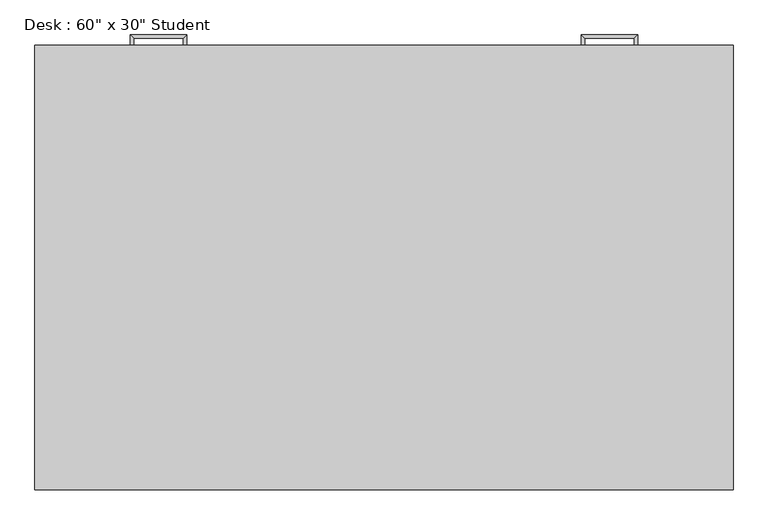
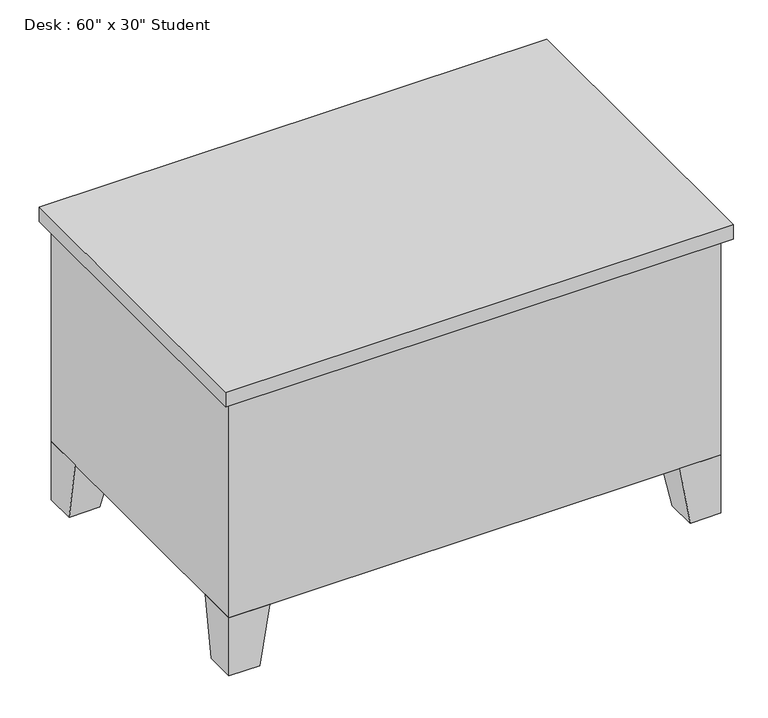
"""IFC4 building model written with IfcOpenShell, lengths in millimetres: furniture geometry."""

from ifc_helpers import new_model, si_unit, frame, origin, place, context, project, spatial, polyline, outline, extrude, faceted_brep, source, transform, mapped, element, save


def furniture_8768a1f0(model_context):
    return source(origin(), model_context, "Body", "SolidModel", [
        extrude(outline(polyline([(1200.15, 762.0), (831.85, 762.0), (831.85, 774.7), (1200.15, 774.7), (1200.15, 762.0)])), frame((0.0, 0.0, 603.25), z_axis=(0.0, 0.0, 1.0), x_axis=(1.0, 0.0, 0.0)), (0.0, 0.0, 1.0), 101.6),
        extrude(outline(polyline([(1200.15, 762.0), (831.85, 762.0), (831.85, 774.7), (1200.15, 774.7), (1200.15, 762.0)])), frame((0.0, 0.0, 171.45), z_axis=(0.0, 0.0, 1.0), x_axis=(1.0, 0.0, 0.0)), (0.0, 0.0, 1.0), 412.75),
        extrude(outline(polyline([(387.35, 762.0), (19.05, 762.0), (19.05, 774.7), (387.35, 774.7), (387.35, 762.0)])), frame((0.0, 0.0, 603.25), z_axis=(0.0, 0.0, 1.0), x_axis=(1.0, 0.0, 0.0)), (0.0, 0.0, 1.0), 101.6),
        extrude(outline(polyline([(387.35, 762.0), (19.05, 762.0), (19.05, 774.7), (387.35, 774.7), (387.35, 762.0)])), frame((0.0, 0.0, 171.45), z_axis=(0.0, 0.0, 1.0), x_axis=(1.0, 0.0, 0.0)), (0.0, 0.0, 1.0), 171.45),
        extrude(outline(polyline([(387.35, 762.0), (19.05, 762.0), (19.05, 774.7), (387.35, 774.7), (387.35, 762.0)])), frame((0.0, 0.0, 482.6), z_axis=(0.0, 0.0, 1.0), x_axis=(1.0, 0.0, 0.0)), (0.0, 0.0, 1.0), 101.6),
        extrude(outline(polyline([(387.35, 762.0), (19.05, 762.0), (19.05, 774.7), (387.35, 774.7), (387.35, 762.0)])), frame((0.0, 0.0, 361.95), z_axis=(0.0, 0.0, 1.0), x_axis=(1.0, 0.0, 0.0)), (0.0, 0.0, 1.0), 101.6),
        faceted_brep([(1117.6, 762.0, 152.4), (1117.6, 660.4, 152.4), (1219.2, 660.4, 152.4), (1219.2, 762.0, 152.4), (1143.0, 762.0, 0.0), (1219.2, 762.0, 0.0), (1219.2, 685.8, 0.0), (1143.0, 685.8, 0.0)], [[[0, 1, 2, 3]], [[4, 5, 6, 7]], [[4, 7, 1, 0]], [[7, 6, 2, 1]], [[6, 5, 3, 2]], [[5, 4, 0, 3]]]),
        faceted_brep([(1117.6, 0.0, 152.4), (1219.2, 0.0, 152.4), (1219.2, 101.6, 152.4), (1117.6, 101.6, 152.4), (1143.0, 0.0, 0.0), (1143.0, 76.2, 0.0), (1219.2, 76.2, 0.0), (1219.2, 0.0, 0.0)], [[[0, 1, 2, 3]], [[4, 5, 6, 7]], [[4, 7, 1, 0]], [[7, 6, 2, 1]], [[6, 5, 3, 2]], [[5, 4, 0, 3]]]),
        faceted_brep([(101.6, 0.0, 152.4), (101.6, 101.6, 152.4), (0.0, 101.6, 152.4), (0.0, 0.0, 152.4), (76.2, 0.0, 0.0), (0.0, 0.0, 0.0), (0.0, 76.2, 0.0), (76.2, 76.2, 0.0)], [[[0, 1, 2, 3]], [[4, 5, 6, 7]], [[4, 7, 1, 0]], [[7, 6, 2, 1]], [[6, 5, 3, 2]], [[5, 4, 0, 3]]]),
        faceted_brep([(101.6, 762.0, 152.4), (0.0, 762.0, 152.4), (0.0, 660.4, 152.4), (101.6, 660.4, 152.4), (76.2, 762.0, 0.0), (76.2, 685.8, 0.0), (0.0, 685.8, 0.0), (0.0, 762.0, 0.0)], [[[0, 1, 2, 3]], [[4, 5, 6, 7]], [[4, 7, 1, 0]], [[7, 6, 2, 1]], [[6, 5, 3, 2]], [[5, 4, 0, 3]]]),
        extrude(outline(polyline([(1238.25, 781.05), (1238.25, -19.05), (-19.05, -19.05), (-19.05, 781.05), (1238.25, 781.05)])), frame((0.0, 0.0, 723.9), z_axis=(0.0, 0.0, 1.0), x_axis=(1.0, 0.0, 0.0)), (0.0, 0.0, 1.0), 38.1),
        extrude(outline(polyline([(406.4, 762.0), (406.4, 50.8), (812.8, 50.8), (812.8, 762.0), (1219.2, 762.0), (1219.2, 0.0), (0.0, 0.0), (0.0, 762.0), (406.4, 762.0)])), frame((0.0, 0.0, 152.4), z_axis=(0.0, 0.0, 1.0), x_axis=(1.0, 0.0, 0.0)), (0.0, 0.0, 1.0), 571.5),
        faceted_brep([(1060.45, 774.7, 546.1), (1060.45, 774.7, 533.4), (1066.8, 774.7, 533.4), (1066.8, 774.7, 546.1), (1060.45, 793.75, 546.1), (1060.45, 793.75, 533.4), (1066.8, 800.1, 533.4), (1066.8, 800.1, 546.1), (971.55, 793.75, 546.1), (971.55, 793.75, 533.4), (965.2, 800.1, 533.4), (965.2, 800.1, 546.1), (971.55, 774.7, 546.1), (965.2, 774.7, 546.1), (965.2, 774.7, 533.4), (971.55, 774.7, 533.4)], [[[0, 1, 2, 3]], [[1, 0, 4, 5]], [[2, 1, 5, 6]], [[3, 2, 6, 7]], [[0, 3, 7, 4]], [[5, 4, 8, 9]], [[6, 5, 9, 10]], [[7, 6, 10, 11]], [[4, 7, 11, 8]], [[12, 13, 14, 15]], [[9, 8, 12, 15]], [[10, 9, 15, 14]], [[11, 10, 14, 13]], [[8, 11, 13, 12]]]),
        faceted_brep([(1060.45, 774.7, 666.75), (1060.45, 774.7, 654.05), (1066.8, 774.7, 654.05), (1066.8, 774.7, 666.75), (1060.45, 793.75, 666.75), (1060.45, 793.75, 654.05), (1066.8, 800.1, 654.05), (1066.8, 800.1, 666.75), (971.55, 793.75, 666.75), (971.55, 793.75, 654.05), (965.2, 800.1, 654.05), (965.2, 800.1, 666.75), (971.55, 774.7, 666.75), (965.2, 774.7, 666.75), (965.2, 774.7, 654.05), (971.55, 774.7, 654.05)], [[[0, 1, 2, 3]], [[1, 0, 4, 5]], [[2, 1, 5, 6]], [[3, 2, 6, 7]], [[0, 3, 7, 4]], [[5, 4, 8, 9]], [[6, 5, 9, 10]], [[7, 6, 10, 11]], [[4, 7, 11, 8]], [[12, 13, 14, 15]], [[9, 8, 12, 15]], [[10, 9, 15, 14]], [[11, 10, 14, 13]], [[8, 11, 13, 12]]]),
        faceted_brep([(158.75, 774.7, 304.8), (152.4, 774.7, 304.8), (152.4, 774.7, 292.1), (158.75, 774.7, 292.1), (158.75, 793.75, 304.8), (152.4, 800.1, 304.8), (152.4, 800.1, 292.1), (158.75, 793.75, 292.1), (247.65, 793.75, 304.8), (254.0, 800.1, 304.8), (254.0, 800.1, 292.1), (247.65, 793.75, 292.1), (247.65, 774.7, 304.8), (247.65, 774.7, 292.1), (254.0, 774.7, 292.1), (254.0, 774.7, 304.8)], [[[0, 1, 2, 3]], [[1, 0, 4, 5]], [[2, 1, 5, 6]], [[3, 2, 6, 7]], [[0, 3, 7, 4]], [[5, 4, 8, 9]], [[6, 5, 9, 10]], [[7, 6, 10, 11]], [[4, 7, 11, 8]], [[12, 13, 14, 15]], [[9, 8, 12, 15]], [[10, 9, 15, 14]], [[11, 10, 14, 13]], [[8, 11, 13, 12]]]),
        faceted_brep([(158.75, 774.7, 425.45), (152.4, 774.7, 425.45), (152.4, 774.7, 412.75), (158.75, 774.7, 412.75), (158.75, 793.75, 425.45), (152.4, 800.1, 425.45), (152.4, 800.1, 412.75), (158.75, 793.75, 412.75), (247.65, 793.75, 425.45), (254.0, 800.1, 425.45), (254.0, 800.1, 412.75), (247.65, 793.75, 412.75), (247.65, 774.7, 425.45), (247.65, 774.7, 412.75), (254.0, 774.7, 412.75), (254.0, 774.7, 425.45)], [[[0, 1, 2, 3]], [[1, 0, 4, 5]], [[2, 1, 5, 6]], [[3, 2, 6, 7]], [[0, 3, 7, 4]], [[5, 4, 8, 9]], [[6, 5, 9, 10]], [[7, 6, 10, 11]], [[4, 7, 11, 8]], [[12, 13, 14, 15]], [[9, 8, 12, 15]], [[10, 9, 15, 14]], [[11, 10, 14, 13]], [[8, 11, 13, 12]]]),
        faceted_brep([(158.75, 774.7, 546.1), (152.4, 774.7, 546.1), (152.4, 774.7, 533.4), (158.75, 774.7, 533.4), (158.75, 793.75, 546.1), (152.4, 800.1, 546.1), (152.4, 800.1, 533.4), (158.75, 793.75, 533.4), (247.65, 793.75, 546.1), (254.0, 800.1, 546.1), (254.0, 800.1, 533.4), (247.65, 793.75, 533.4), (247.65, 774.7, 546.1), (247.65, 774.7, 533.4), (254.0, 774.7, 533.4), (254.0, 774.7, 546.1)], [[[0, 1, 2, 3]], [[1, 0, 4, 5]], [[2, 1, 5, 6]], [[3, 2, 6, 7]], [[0, 3, 7, 4]], [[5, 4, 8, 9]], [[6, 5, 9, 10]], [[7, 6, 10, 11]], [[4, 7, 11, 8]], [[12, 13, 14, 15]], [[9, 8, 12, 15]], [[10, 9, 15, 14]], [[11, 10, 14, 13]], [[8, 11, 13, 12]]]),
        faceted_brep([(158.75, 774.7, 666.75), (152.4, 774.7, 666.75), (152.4, 774.7, 654.05), (158.75, 774.7, 654.05), (158.75, 793.75, 666.75), (152.4, 800.1, 666.75), (152.4, 800.1, 654.05), (158.75, 793.75, 654.05), (247.65, 793.75, 666.75), (254.0, 800.1, 666.75), (254.0, 800.1, 654.05), (247.65, 793.75, 654.05), (247.65, 774.7, 666.75), (247.65, 774.7, 654.05), (254.0, 774.7, 654.05), (254.0, 774.7, 666.75)], [[[0, 1, 2, 3]], [[1, 0, 4, 5]], [[2, 1, 5, 6]], [[3, 2, 6, 7]], [[0, 3, 7, 4]], [[5, 4, 8, 9]], [[6, 5, 9, 10]], [[7, 6, 10, 11]], [[4, 7, 11, 8]], [[12, 13, 14, 15]], [[9, 8, 12, 15]], [[10, 9, 15, 14]], [[11, 10, 14, 13]], [[8, 11, 13, 12]]]),
    ])


if __name__ == "__main__":
    model = new_model("IFC4")
    model_context = context("Model", 3, world=origin())
    ifc_project = project(units=[si_unit("LENGTHUNIT", "METRE", prefix="MILLI")], contexts=[model_context])
    site = spatial("IfcSite", under=ifc_project)
    building = spatial("IfcBuilding", under=site)
    placement = place(None, origin())
    furniture_shape = furniture_8768a1f0(model_context)
    element("IfcFurniture", 1, ObjectType="Desk : 60\" x 30\" Student", at=placement, inside=building, context=model_context, shape_type="MappedRepresentation", body=[
        mapped(furniture_shape, transform((0.0, 0.0, 0.0), x_axis=(1.0, 0.0, 0.0), y_axis=(0.0, 1.0, 0.0), z_axis=(0.0, 0.0, 1.0))),
    ])
    save(model, "model.ifc")

# Revit data of these elements
# Type "Desk : 60\" x 30\" Student"
#   Assembly Code = "E2020200"
#   Depth = 2' - 6"
#   Height = 2' - 6"
#   Leg Height = 0' - 6"
#   Width = 4' - 0"
#   Body Material = Laminate, Ivory, Matte
#   Handle/Leg Material = Steel, Chrome Plated
#   Top Material = Cherry
#   Default Elevation = 0
# Element 1 (IfcFurniture, "Desk : 60\" x 30\" Student")
#   Materials on its faces: "Steel, Chrome Plated", "Laminate, Ivory, Matte", "Cherry"
# Materials
#   "Laminate, Ivory, Matte": class "Plastic", colour RGB 247 247 239, transparency 0, Description = "Plastic Laminate - Ivory, Matte", Cost = 0
#   "Steel, Chrome Plated": class "Metal", colour RGB 17 17 17, transparency 0, Description = "Chromiuim plated steel", Cost = 0
#   "Cherry": class "Wood", colour RGB 226 177 128, transparency 0, Description = "Prunus Serotina", Cost = 0
